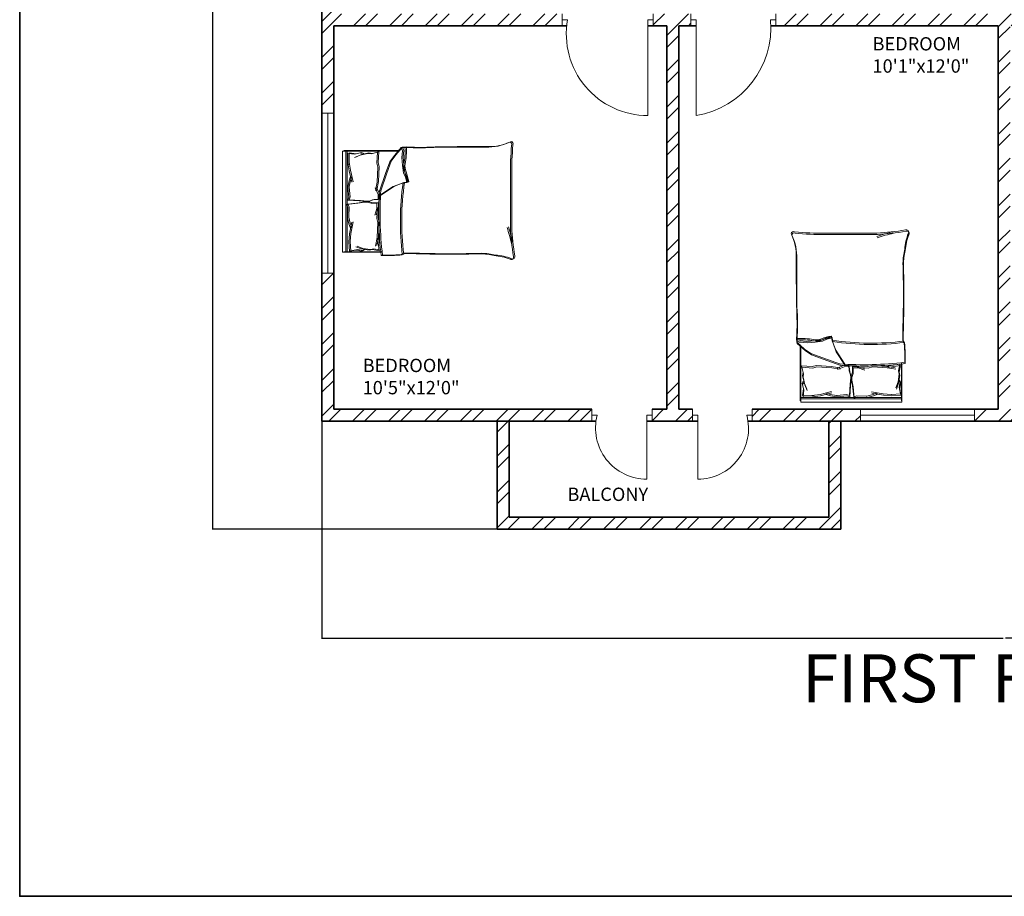
# Model space of a CAD drawing. Units: inches. Extents: x 1944 to 3454, y 1352 to 3055.
# Tile 1 of 17: x 1944 to 2314, y 1352 to 1681. Entities that reach past the tile are written whole.
import ezdxf

# ---------------------------------------------------------------- set-up
doc = ezdxf.new("R2010")
doc.units = ezdxf.units.IN
for name, color, linetype, lineweight in [('A-ANNO-DIMS', 2, 'Continuous', 18), ('A-ANNO-TITL', 7, 'Continuous', 30), ('A-ANNO-TTLB', 7, 'Continuous', 35), ('A-AREA-IDEN', 7, 'Continuous', 18), ('A-DOOR', 3, 'Continuous', 20), ('A-FURN', 8, 'Continuous', 13), ('A-GLAZ', 4, 'Continuous', 18), ('A-WALL', 7, 'Continuous', 35), ('A-WALL-PATT', 252, 'Continuous', 13)]:
    doc.layers.add(name, color=color, linetype=linetype, lineweight=lineweight)
doc.styles.get("Standard").update_dxf_attribs({"font": 'arial.ttf'})
doc.dimstyles.get("Standard").update_dxf_attribs({"dimtxt": 0.18, "dimasz": 0.18, "dimexe": 0.18, "dimexo": 0.0625, "dimgap": 0.09, "dimtad": 0, "dimtih": 1, "dimtoh": 1, "dimdec": 4, "dimzin": 0, "dimdsep": 46, "dimtxsty": 'Standard', "dimcen": 0.09, "dimadec": 0, "dimazin": 0, "dimtfac": 1, "dimtdec": 4, "dimtofl": 0, "dimtmove": 0, "dimatfit": 3, "dimfxl": 1, "dimtolj": 1, "dimtzin": 0, "dimarcsym": 0})

# ---------------------------------------------------------------- blocks, each defined once
blk = doc.blocks.new('BED-WITH-PILLOWS-01')
for p, q in [((0, 40.75), (21.15, 40.75)), ((0, 40.75), (21.15, 40.75)), ((0, 2.76), (0, 40.75)), ((0.51, 40.93), (21.66, 40.93)), ((0.51, 40.93), (21.66, 40.93)), ((1.22, 2.76), (1.22, 40.75)), ((1.22, 2.76), (1.22, 40.75)), ((1.73, 2.94), (1.73, 40.93)), ((1.73, 2.94), (1.73, 40.93)), ((22.05, 42.02), (19.47, 39.08)), ((22.05, 42.02), (19.47, 39.08)), ((22.56, 42.21), (19.98, 39.26)), ((22.56, 42.21), (19.98, 39.26)), ((23.44, 42.09), (22.05, 42.02, 3.08)), ((23.44, 42.09), (22.05, 42.02, 3.08)), ((22.55, 40.8), (22.05, 42.02)), ((22.55, 40.8), (22.05, 42.02)), ((22.3, 38.34), (22.55, 40.8)), ((22.3, 38.34), (22.55, 40.8)), ((23.95, 42.27), (22.56, 42.21, 3.08)), ((23.95, 42.27), (22.56, 42.21, 3.08)), ((23.05, 40.98), (22.56, 42.21)), ((23.05, 40.98), (22.56, 42.21)), ((22.81, 38.52), (23.05, 40.98)), ((22.81, 38.52), (23.05, 40.98)), ((2.03, 39.83), (1.96, 35.54)), ((2.03, 39.83), (1.96, 35.54)), ((2.03, 39.83), (4.58, 39.53)), ((2.03, 39.83), (4.58, 39.53)), ((2.54, 40.01), (2.46, 35.72)), ((2.54, 40.01), (2.46, 35.72)), ((2.54, 40.01), (5.09, 39.71)), ((2.54, 40.01), (5.09, 39.71)), ((6.56, 39.2), (4.43, 38.26)), ((6.56, 39.2), (4.43, 38.26)), ((4.58, 39.53), (6.63, 40.01)), ((4.58, 39.53), (6.63, 40.01)), ((7.07, 39.38), (4.94, 38.44)), ((7.07, 39.38), (4.94, 38.44)), ((5.09, 39.71), (7.14, 40.19)), ((5.09, 39.71), (7.14, 40.19)), ((9.4, 39.83), (6.56, 39.2)), ((9.4, 39.83), (6.56, 39.2)), ((6.63, 40.01), (7.46, 39.6)), ((6.63, 40.01), (7.46, 39.6)), ((9.91, 40.01), (7.07, 39.38)), ((9.91, 40.01), (7.07, 39.38)), ((7.14, 40.19), (7.97, 39.78)), ((7.14, 40.19), (7.97, 39.78)), ((10.68, 39.68), (9.4, 39.83)), ((10.68, 39.68), (9.4, 39.83)), ((11.19, 39.86), (9.91, 40.01)), ((11.19, 39.86), (9.91, 40.01)), ((13.17, 40.3), (10.68, 39.68)), ((13.17, 40.3), (10.68, 39.68)), ((13.68, 40.48), (11.19, 39.86)), ((13.68, 40.48), (11.19, 39.86)), ((12.85, 36.22), (13.17, 40.3)), ((12.85, 36.22), (13.17, 40.3)), ((13.36, 36.4), (13.68, 40.48)), ((13.36, 36.4), (13.68, 40.48)), ((19.47, 39.08), (17.75, 36.74)), ((19.47, 39.08), (17.75, 36.74)), ((19.98, 39.26), (18.26, 36.92)), ((19.98, 39.26), (18.26, 36.92)), ((22.55, 35.26), (22.3, 38.34)), ((22.55, 35.26), (22.3, 38.34)), ((23.05, 35.44), (22.81, 38.52)), ((23.05, 35.44), (22.81, 38.52)), ((1.96, 35.54), (2.02, 36.34)), ((1.96, 35.54), (2.02, 36.34)), ((2.02, 36.34), (2.44, 33.32)), ((2.02, 36.34), (2.44, 33.32)), ((2.44, 33.32), (3.51, 29.01)), ((2.44, 33.32), (3.51, 29.01)), ((2.46, 35.72), (2.53, 36.52)), ((2.46, 35.72), (2.53, 36.52)), ((2.53, 36.52), (2.95, 33.5)), ((2.53, 36.52), (2.95, 33.5)), ((2.95, 33.5), (4.02, 29.19)), ((2.95, 33.5), (4.02, 29.19)), ((13.3, 34.66), (12.85, 36.22)), ((13.3, 34.66), (12.85, 36.22)), ((12.95, 29.09), (13.3, 34.66)), ((12.95, 29.09), (13.3, 34.66)), ((13.8, 34.84), (13.36, 36.4)), ((13.8, 34.84), (13.36, 36.4)), ((13.46, 29.27), (13.8, 34.84)), ((13.46, 29.27), (13.8, 34.84)), ((17.75, 36.74), (16.15, 32.31)), ((17.75, 36.74), (16.15, 32.31)), ((18.26, 36.92), (16.66, 32.49)), ((18.26, 36.92), (16.66, 32.49)), ((22.92, 32.55), (22.55, 35.26)), ((22.92, 32.55), (22.55, 35.26)), ((23.42, 32.74), (23.05, 35.44)), ((23.42, 32.74), (23.05, 35.44)), ((2.92, 31.16), (2.45, 29.52)), ((2.92, 31.16), (2.45, 29.52)), ((2.95, 29.7), (2.52, 27.37)), ((2.95, 29.7), (2.52, 27.37)), ((3.43, 31.34), (2.95, 29.7)), ((3.43, 31.34), (2.95, 29.7)), ((16.15, 32.31), (13.82, 25.68)), ((16.15, 32.31), (13.82, 25.68)), ((16.66, 32.49), (14.33, 25.86)), ((16.66, 32.49), (14.33, 25.86)), ((23.65, 30.95), (22.92, 32.55)), ((23.65, 30.95), (22.92, 32.55)), ((24.16, 31.13), (23.42, 32.74)), ((24.16, 31.13), (23.42, 32.74)), ((24.15, 28.98), (23.65, 30.95)), ((24.15, 28.98), (23.65, 30.95)), ((24.65, 29.17), (24.16, 31.13)), ((24.65, 29.16), (24.16, 31.13)), ((62.99, 11.97), (62.99, 31.54)), ((62.99, 11.97), (62.99, 31.54)), ((63.5, 12.16), (63.5, 31.72)), ((63.5, 12.15), (63.5, 31.72)), ((2.45, 29.52), (2.02, 27.19)), ((2.45, 29.52), (2.02, 27.19)), ((2.02, 27.19), (2.03, 26.93)), ((2.02, 27.19), (2.03, 26.93)), ((2.03, 26.93), (2.37, 23.41)), ((2.03, 26.93), (2.37, 23.41)), ((2.52, 27.37), (2.54, 27.12)), ((2.52, 27.37), (2.54, 27.11)), ((2.54, 27.12), (2.88, 23.6)), ((2.54, 27.11), (2.88, 23.6)), ((13.31, 24.44), (12.28, 26.88)), ((13.31, 24.44), (12.28, 26.88)), ((12.42, 25.88), (12.95, 29.09)), ((12.42, 25.88), (12.95, 29.09)), ((13.81, 24.62), (12.79, 27.07)), ((13.81, 24.62), (12.79, 27.06)), ((12.93, 26.07), (13.46, 29.27)), ((12.93, 26.07), (13.46, 29.27)), ((13.82, 24.05), (18.98, 27.38)), ((13.82, 24.05), (18.98, 27.38)), ((14.33, 24.23), (19.49, 27.56)), ((14.33, 24.23), (19.49, 27.56)), ((18.98, 27.38), (22.55, 28.74)), ((18.98, 27.38), (22.55, 28.74)), ((19.49, 27.56), (23.05, 28.92)), ((19.49, 27.56), (23.05, 28.92)), ((22.55, 28.74), (24.15, 28.98)), ((22.55, 28.74), (24.15, 28.98)), ((23.05, 28.92), (24.65, 29.17)), ((23.05, 28.92), (24.65, 29.16)), ((2.37, 23.41), (1.98, 22.24)), ((2.37, 23.41), (1.98, 22.24)), ((1.98, 22.24), (6.25, 22.04)), ((1.98, 22.24), (6.25, 22.04)), ((2.88, 23.6), (2.49, 22.42)), ((2.88, 23.6), (2.49, 22.42)), ((2.49, 22.42), (6.76, 22.23)), ((2.49, 22.42), (6.76, 22.23)), ((6.76, 22.23), (9.31, 21.93)), ((6.76, 22.23), (9.31, 21.93)), ((9.84, 21.81), (11.3, 22.36)), ((9.84, 21.81), (11.3, 22.36)), ((10.35, 21.99), (11.81, 22.54)), ((10.35, 21.99), (11.81, 22.54)), ((11.3, 22.36), (13.43, 22.49)), ((11.3, 22.36), (13.43, 22.49)), ((11.81, 22.54), (13.94, 22.67)), ((11.81, 22.54), (13.94, 22.67)), ((13.43, 22.49), (13.31, 24.44)), ((13.43, 22.49), (13.31, 24.44)), ((13.94, 22.67), (13.81, 24.62)), ((13.94, 22.67), (13.81, 24.62)), ((1.49, 20.65), (5.74, 21.11)), ((1.49, 20.65), (5.74, 21.11)), ((1.95, 19.5), (1.49, 20.65)), ((1.95, 19.5), (1.49, 20.65)), ((1.83, 15.97), (1.95, 19.5)), ((1.83, 15.97), (1.95, 19.5)), ((1.99, 20.83), (6.25, 21.29)), ((1.99, 20.83), (6.25, 21.29)), ((2.45, 19.69), (1.99, 20.83)), ((2.45, 19.69), (1.99, 20.83)), ((2.34, 16.15), (2.45, 19.69)), ((2.34, 16.15), (2.45, 19.69)), ((5.74, 21.11), (8.27, 21.57)), ((5.74, 21.11), (8.27, 21.57)), ((6.25, 22.04), (8.81, 21.74)), ((6.25, 22.04), (8.81, 21.74)), ((6.25, 21.29), (8.78, 21.75)), ((6.25, 21.29), (8.78, 21.75)), ((8.27, 21.57), (9.3, 21.57)), ((8.27, 21.57), (9.3, 21.57)), ((8.78, 21.75), (9.81, 21.75)), ((8.78, 21.75), (9.81, 21.75)), ((8.81, 21.74), (9.84, 21.81)), ((8.81, 21.74), (9.84, 21.81)), ((9.3, 21.57), (10.8, 21.11)), ((9.3, 21.57), (10.8, 21.11)), ((9.31, 21.93), (10.35, 21.99)), ((9.31, 21.93), (10.35, 21.99)), ((9.81, 21.75), (11.3, 21.29)), ((9.81, 21.75), (11.3, 21.29)), ((10.8, 21.11), (12.93, 21.11)), ((10.8, 21.11), (12.93, 21.11)), ((11.3, 21.29), (13.44, 21.29)), ((11.3, 21.29), (13.44, 21.29)), ((12.93, 19.16), (12.06, 16.66)), ((12.93, 19.16), (12.06, 16.66)), ((13.44, 19.34), (12.57, 16.84)), ((13.44, 19.34), (12.57, 16.84)), ((12.85, 15.41), (13.17, 19.49)), ((12.85, 15.41), (13.17, 19.49)), ((12.93, 21.11), (12.93, 19.16)), ((12.93, 21.11), (12.93, 19.16)), ((13.36, 15.59), (13.68, 19.67)), ((13.36, 15.59), (13.68, 19.67)), ((13.44, 21.29), (13.44, 19.34)), ((13.44, 21.29), (13.44, 19.34)), ((1.83, 15.71), (1.83, 15.97)), ((1.83, 15.71), (1.83, 15.97)), ((2.41, 13.42), (1.83, 15.71)), ((2.41, 13.42), (1.83, 15.71)), ((2.34, 15.9), (2.34, 16.15)), ((2.34, 15.9), (2.34, 16.15)), ((2.91, 13.6), (2.34, 15.9)), ((2.91, 13.6), (2.34, 15.9)), ((13.3, 13.85), (12.85, 15.41)), ((13.3, 13.85), (12.85, 15.41)), ((13.8, 14.03), (13.36, 15.59)), ((13.8, 14.03), (13.36, 15.59)), ((2.98, 11.81), (2.41, 13.42)), ((2.98, 11.81), (2.41, 13.42)), ((2.64, 9.62), (3.44, 13.99)), ((2.64, 9.62), (3.44, 13.99)), ((3.49, 11.99), (2.91, 13.6)), ((3.49, 11.99), (2.91, 13.6)), ((3.14, 9.81), (3.95, 14.17)), ((3.14, 9.81), (3.95, 14.17)), ((12.95, 8.28), (13.3, 13.85)), ((12.95, 8.28), (13.3, 13.85)), ((13.46, 8.46), (13.8, 14.03)), ((13.46, 8.46), (13.8, 14.03)), ((2.41, 6.59), (2.64, 9.62)), ((2.41, 6.59), (2.64, 9.62)), ((2.91, 6.77), (3.14, 9.81)), ((2.91, 6.77), (3.14, 9.81)), ((12.42, 5.07), (12.95, 8.28)), ((12.42, 5.07), (12.95, 8.28)), ((12.93, 5.25), (13.46, 8.46)), ((12.93, 5.25), (13.46, 8.46)), ((12.95, 8.28), (13.21, 7.38)), ((12.95, 8.28), (13.21, 7.38)), ((13.46, 8.46), (13.72, 7.56)), ((13.46, 8.46), (13.72, 7.56)), ((13.72, 7.56), (14.29, 3.51)), ((13.72, 7.56), (14.29, 3.51)), ((2.39, 6.5), (2.41, 6.59)), ((2.39, 6.5), (2.41, 6.59)), ((2.65, 3.1), (2.39, 6.5)), ((2.65, 3.1), (2.39, 6.5)), ((2.9, 6.68), (2.91, 6.77)), ((2.9, 6.68), (2.91, 6.77)), ((3.16, 3.28), (2.9, 6.68)), ((3.16, 3.28), (2.9, 6.68)), ((3.14, 3.28), (5.67, 3.74)), ((3.14, 3.28), (5.67, 3.74)), ((7.12, 4.02), (4.93, 4.82)), ((7.12, 4.01), (4.93, 4.82)), ((7.63, 4.2), (5.44, 5)), ((7.63, 4.2), (5.44, 5)), ((5.67, 3.74), (7.74, 3.39)), ((5.67, 3.74), (7.74, 3.39)), ((9.99, 3.56), (7.12, 4.02)), ((9.99, 3.56), (7.12, 4.01)), ((10.5, 3.74), (7.63, 4.2)), ((10.5, 3.74), (7.63, 4.2)), ((7.74, 3.39), (8.55, 3.85)), ((7.74, 3.39), (8.55, 3.85)), ((11.26, 3.79), (9.99, 3.56)), ((11.26, 3.79), (9.99, 3.56)), ((11.76, 3.97), (10.5, 3.74)), ((11.76, 3.97), (10.5, 3.74)), ((13.78, 3.33), (11.26, 3.79)), ((13.78, 3.33), (11.26, 3.79)), ((14.29, 3.51), (11.76, 3.97)), ((14.29, 3.51), (11.76, 3.97)), ((13.21, 7.38), (13.78, 3.33)), ((13.21, 7.38), (13.78, 3.33)), ((14.4, 2.76), (0, 2.76)), ((14.4, 2.76), (0, 2.76)), ((14.9, 2.94), (0.51, 2.94)), ((14.9, 2.94), (0.51, 2.94)), ((2.64, 3.1), (5.16, 3.56)), ((2.64, 3.1), (5.16, 3.56)), ((5.16, 3.56), (7.23, 3.21)), ((5.16, 3.56), (7.23, 3.21)), ((7.23, 3.21), (8.04, 3.67)), ((7.23, 3.21), (8.04, 3.67))]:
    blk.add_line(p, q)
for centre, radius, start, end in [((-5.29, 40.8), 28.76, 349.8763, 2.5657), ((-5.29, 40.8), 28.76, 349.8763, 2.5657), ((28.87, 144.88), 102.94, 266.9791, 273.8365), ((28.87, 144.88), 102.94, 266.9791, 273.8365), ((-4.78, 40.98), 28.76, 349.8763, 2.5657), ((-4.78, 40.98), 28.76, 349.8763, 2.5657), ((29.37, 145.06), 102.94, 266.9791, 273.8365), ((29.37, 145.06), 102.94, 266.9791, 273.8365), ((53.91, -3583.94), 3626.16, 90.00217, 90.28689), ((53.91, -3583.94), 3626.16, 90.00217, 90.28689), ((54.42, -3583.76), 3626.16, 90.00217, 90.28689), ((54.42, -3583.76), 3626.16, 90.00217, 90.28689), ((54.58, 60.54), 18.33, 267.4714, 296.4681), ((54.58, 60.54), 18.33, 267.4714, 296.4681), ((55.09, 60.72), 18.33, 267.4714, 296.4681), ((55.09, 60.72), 18.33, 267.4714, 296.4681), ((62.69, 43.25), 0.876, 332.6588, 86.02), ((62.69, 43.25), 0.876, 332.6588, 86.02), ((168.74, 32.71), 105.75, 174.4998, 180.6351), ((168.74, 32.71), 105.75, 174.4998, 180.6351), ((63.2, 43.43), 0.876, 332.6588, 86.02), ((63.2, 43.43), 0.876, 332.6588, 86.02), ((169.24, 32.89), 105.75, 174.4998, 180.6351), ((169.24, 32.89), 105.75, 174.4998, 180.6351), ((27.87, 34.77), 4.95, 168.6608, 203.7384), ((27.87, 34.77), 4.95, 168.6608, 203.7384), ((28.38, 34.95), 4.95, 168.6608, 203.7384), ((28.38, 34.95), 4.95, 168.6608, 203.7384), ((1.18, 24.76), 23.57, 10.6617, 19.8806), ((1.18, 24.76), 23.57, 10.6617, 19.8806), ((1.69, 24.95), 23.57, 10.6617, 19.8806), ((1.69, 24.94), 23.57, 10.6617, 19.8806), ((144.71, 16.98), 131.13, 176.0865, 186.7821), ((144.71, 16.98), 131.13, 176.0865, 186.7821), ((145.22, 17.16), 131.13, 176.0865, 186.7821), ((145.22, 17.16), 131.13, 176.0865, 186.7821), ((124.25, 14.11), 102.56, 171.7845, 186.9006), ((124.25, 14.11), 102.56, 171.7845, 186.9006), ((124.76, 14.3), 102.56, 171.7845, 186.9006), ((124.76, 14.3), 102.56, 171.7845, 186.9006), ((24.2, 29.12), 0.147, 250.2464, 1.1377), ((24.2, 29.12), 0.147, 250.2464, 1.1377), ((24.7, 29.3), 0.147, 250.2464, 1.1377), ((24.7, 29.3), 0.147, 250.2464, 1.1377), ((-18.85, -13.69), 84.62, 13.3832, 17.7053), ((-18.85, -13.69), 84.62, 13.3832, 17.7053), ((-18.34, -13.51), 84.62, 13.3832, 17.7053), ((-18.34, -13.51), 84.62, 13.3832, 17.7053), ((159.64, 17.03), 96.78, 182.9958, 189.4091), ((159.64, 17.03), 96.78, 182.9958, 189.4091), ((160.15, 17.21), 96.78, 182.9958, 189.4091), ((160.15, 17.21), 96.78, 182.9958, 189.4091), ((15.97, 67.69), 66.22, 268.7218, 275.604), ((15.97, 67.69), 66.22, 268.7218, 275.604), ((16.48, 67.88), 66.22, 268.7218, 275.604), ((16.48, 67.88), 66.22, 268.7218, 275.604), ((24.78, -132.99), 135.22, 88.4762, 91.0082), ((24.78, -132.99), 135.22, 88.4762, 91.0082), ((25.29, -132.81), 135.22, 88.4762, 91.0082), ((25.29, -132.81), 135.22, 88.4762, 91.0082), ((40.23, 385.38), 383.38, 268.2277, 271.7185), ((40.23, 385.38), 383.38, 268.2277, 271.7185), ((40.74, 385.56), 383.38, 268.2277, 271.7185), ((40.74, 385.56), 383.38, 268.2277, 271.7185), ((51.28, -21.38), 23.56, 76.0648, 88.9113), ((51.28, -21.38), 23.56, 76.0648, 88.9113), ((51.79, -21.2), 23.56, 76.0648, 88.9113), ((51.79, -21.2), 23.56, 76.0648, 88.9113), ((55.86, -17.22), 18.73, 67.9751, 86.652), ((55.86, -17.22), 18.73, 67.9751, 86.652), ((56.37, -17.04), 18.73, 67.9751, 86.652), ((56.37, -17.04), 18.73, 67.9751, 86.652), ((63.37, 0.86), 0.866, 236.1736, 23.4781), ((63.37, 0.86), 0.866, 236.1736, 23.4781), ((63.87, 1.05), 0.866, 236.1736, 23.4781), ((63.87, 1.05), 0.866, 236.1736, 23.4781)]:
    blk.add_arc(centre, radius, start, end)
blk = doc.blocks.new('DOOR-SWING-36IN-07')
for p, q in [((0, 38.25), (0, 33.75)), ((34.17, 33.75), (34.17, 38.25)), ((34.17, 38.25), (34.17, 36)), ((0, 33.75), (0, 36)), ((0, 36), (2, 36)), ((34.17, 36), (32.17, 36)), ((32.17, 36), (32.17, 0))]:
    blk.add_line(p, q)
blk.add_arc((32.17, 30.64), 30.64, 169.9223, 270)
blk = doc.blocks.new('DOOR-SWING-36IN-08')
for p, q in [((0, 33.75), (0, 38.25)), ((0, 38.25), (0, 38.25)), ((0, 38.25), (0, 36)), ((31.9, 38.25), (31.9, 33.75)), ((0, 36), (2, 36)), ((2, 36), (2, 0)), ((31.9, 36), (29.9, 36)), ((31.9, 33.75), (31.9, 36))]:
    blk.add_line(p, q)
blk.add_arc((-3.46, 33.05), 33.5, 279.3869, 5.0549)
blk = doc.blocks.new('DOOR-SWING-24IN-09')
for p, q in [((0, 21.75), (0, 26.25)), ((0, 26.25), (0, 24)), ((22.65, 26.25), (22.65, 21.75)), ((0, 24), (2, 24)), ((22.65, 24), (20.65, 24)), ((20.65, 24), (20.65, 0)), ((22.65, 21.75), (22.65, 24)), ((22.65, 21.75), (22.65, 21.75))]:
    blk.add_line(p, q)
blk.add_arc((20.65, 19.25), 19.25, 165.7058, 270)
blk = doc.blocks.new('DOOR-SWING-24IN-10')
for p, q in [((0, 26.25), (0, 21.75)), ((22.35, 21.75), (22.35, 26.25)), ((22.35, 26.25), (22.35, 24)), ((0, 21.75), (0, 24)), ((0, 24), (2, 24)), ((2, 24), (2, 0)), ((22.35, 24), (20.35, 24))]:
    blk.add_line(p, q)
blk.add_arc((2, 19.01), 19.01, 270, 15.2011)
blk = doc.blocks.new('WINDOW-PLAN-60.00IN-02')
for p, q in [((2.25, 60), (0, 60)), ((0, 60), (4.5, 60)), ((2.25, 0), (2.25, 60)), ((0, 0), (4.5, 0)), ((4.5, 0), (2.25, 0))]:
    blk.add_line(p, q)
blk = doc.blocks.new('WINDOW-PLAN-42.86IN-01')
for p, q in [((0, 4.5), (0, 0)), ((42.86, 2.25), (42.86, 4.5)), ((42.86, 4.5), (42.86, 0)), ((0, 0), (0, 2.25)), ((0, 2.25), (42.86, 2.25))]:
    blk.add_line(p, q)
blk = doc.blocks.new('*D184')
at = {"layer": 'A-ANNO-DIMS', "color": 0, "lineweight": -2, "transparency": 16777216}
for p, q in [((2057.32, 1530.03), (2057.32, 1448.47)), ((2569.82, 1530.03), (2569.82, 1448.47)), ((2057.5, 1448.65), (2313.18, 1448.65)), ((2569.64, 1448.65), (2313.97, 1448.65))]:
    blk.add_line(p, q, dxfattribs=at)
at = {"layer": 'A-ANNO-DIMS', "color": 0, "transparency": 16777216}
for points in [[(2057.5, 1448.68), (2057.5, 1448.62), (2057.32, 1448.65)], [(2569.64, 1448.68), (2569.64, 1448.62), (2569.82, 1448.65)]]:
    blk.add_solid(points, dxfattribs=at)
at = {"layer": 'Defpoints', "color": 0, "transparency": 16777216}
for p in [(2057.32, 1530.1), (2569.82, 1530.1), (2569.82, 1448.65)]:
    blk.add_point(p, dxfattribs=at)
at = {"layer": 'A-ANNO-DIMS', "color": 0, "transparency": 16777216, "insert": (2313.57, 1448.65), "char_height": 0.18, "attachment_point": 5}
blk.add_mtext('\\A1;512.5', dxfattribs=at)
blk = doc.blocks.new('*D185')
at = {"layer": 'A-ANNO-DIMS', "color": 0, "lineweight": -2, "transparency": 16777216}
for p, q in [((2122.1, 2222.6), (2016.19, 2222.6)), ((2016.37, 2222.42), (2016.37, 1856.28)), ((2016.37, 1489.78), (2016.37, 1855.91)), ((2123.11, 1489.6), (2016.19, 1489.6))]:
    blk.add_line(p, q, dxfattribs=at)
at = {"layer": 'A-ANNO-DIMS', "color": 0, "transparency": 16777216}
for points in [[(2016.34, 2222.42), (2016.4, 2222.42), (2016.37, 2222.6)], [(2016.34, 1489.78), (2016.4, 1489.78), (2016.37, 1489.6)]]:
    blk.add_solid(points, dxfattribs=at)
at = {"layer": 'Defpoints', "color": 0, "transparency": 16777216}
for p in [(2016.37, 2222.6), (2122.17, 2222.6), (2123.17, 1489.6)]:
    blk.add_point(p, dxfattribs=at)
at = {"layer": 'A-ANNO-DIMS', "color": 0, "transparency": 16777216, "insert": (2016.37, 1856.1), "char_height": 0.18, "attachment_point": 5}
blk.add_mtext('\\A1;733', dxfattribs=at)

msp = doc.modelspace()

# ---------------------------------------------------------------- hatches: boundary and pattern name
at = {"layer": 'A-WALL-PATT'}
h = msp.add_hatch(dxfattribs=at)
h.set_pattern_fill('ANSI32', color=256)
h.paths.add_polyline_path([(2061.822, 2177.596), (2158.181, 2177.596), (2158.181, 2179.846), (2158.181, 2182.096), (2057.322, 2182.096), (2057.322, 2123.452), (2061.822, 2123.452)])
h.paths.add_polyline_path([(2258.993, 2179.846), (2258.993, 2182.096), (2218.838, 2182.096), (2218.838, 2177.596), (2258.993, 2177.596)])
h.paths.add_polyline_path([(2315.822, 2177.596), (2322.722, 2177.596), (2322.722, 2182.096), (2303.186, 2182.096), (2303.186, 2177.596), (2311.322, 2177.596), (2311.322, 2033.596), (2231.355, 2033.596), (2231.355, 2029.096), (2311.322, 2029.096), (2311.322, 1904.596), (2307.941, 1904.596), (2307.941, 1900.096), (2319.277, 1900.096), (2319.277, 1902.346), (2319.277, 1904.596), (2315.822, 1904.596), (2315.822, 2029.096), (2394.855, 2029.096), (2394.855, 2033.596), (2315.822, 2033.596)])
h.paths.add_polyline_path([(2407.334, 2182.096), (2366.1, 2182.096), (2366.1, 2177.596), (2407.334, 2177.596), (2407.334, 2179.846)])
h.paths.add_polyline_path([(2440.322, 2177.596), (2443.866, 2177.596), (2443.866, 2182.096), (2431.827, 2182.096), (2431.827, 2179.846), (2431.827, 2177.596), (2435.822, 2177.596), (2435.822, 2033.596), (2430.464, 2033.596), (2430.464, 2029.096), (2445.372, 2029.096), (2445.372, 2031.346), (2445.372, 2033.596), (2440.322, 2033.596)])
h.paths.add_polyline_path([(2569.822, 2182.096), (2466.481, 2182.096), (2466.481, 2177.596), (2565.322, 2177.596), (2565.322, 2123.452), (2569.822, 2123.452)])
h.paths.add_polyline_path([(2569.822, 2063.452), (2567.572, 2063.452), (2565.322, 2063.452), (2565.322, 2033.596), (2478.08, 2033.596), (2476.822, 2033.596), (2476.822, 2028.698), (2476.822, 2020.069), (2481.322, 2020.069), (2481.322, 2029.096), (2565.322, 2029.096), (2565.322, 2014.5), (2569.822, 2014.5)])
h.paths.add_polyline_path([(2569.822, 1978.5), (2565.322, 1978.5), (2565.322, 1957.096), (2481.322, 1957.096), (2481.322, 1990.369), (2476.822, 1990.369), (2476.822, 1957.096), (2476.822, 1952.596), (2476.822, 1947.471), (2481.322, 1947.471), (2481.322, 1952.596), (2565.322, 1952.596), (2565.322, 1943.2), (2569.822, 1943.2)])
h.paths.add_polyline_path([(2569.822, 1919.2), (2565.322, 1919.2), (2565.322, 1904.596), (2481.322, 1904.596), (2481.322, 1928.596), (2476.822, 1928.596), (2476.822, 1904.596), (2350.518, 1904.596), (2350.518, 1900.096), (2476.822, 1900.096), (2565.322, 1900.096), (2565.322, 1895.596), (2565.322, 1887.047), (2569.822, 1887.047)])
h.paths.add_polyline_path([(2280.492, 1904.596), (2150.322, 1904.596), (2150.322, 1926.68), (2148.072, 1926.68), (2145.822, 1926.68), (2145.822, 1904.596), (2061.822, 1904.596), (2061.822, 1914.977), (2059.572, 1914.977), (2057.322, 1914.977), (2057.322, 1887.362), (2061.822, 1887.362), (2061.822, 1900.096), (2150.322, 1900.096), (2280.492, 1900.096), (2280.492, 1902.346)])
h.paths.add_polyline_path([(2150.322, 1957.096), (2150.322, 1986.22), (2145.822, 1986.22), (2145.822, 1957.096), (2061.822, 1957.096), (2061.822, 1975.678), (2057.322, 1975.678), (2057.322, 1938.977), (2061.822, 1938.977), (2061.822, 1952.596), (2145.822, 1952.596), (2145.822, 1947.985), (2150.322, 1947.985), (2150.322, 1952.596)])
h.paths.add_polyline_path([(2061.822, 2063.452), (2057.322, 2063.452), (2057.322, 2011.678), (2061.822, 2011.678), (2061.822, 2029.096), (2145.288, 2029.096), (2145.822, 2029.096), (2145.822, 2019.118), (2150.322, 2019.118), (2150.322, 2029.096), (2150.322, 2033.596), (2147.022, 2033.596), (2061.822, 2033.596)])
h.paths.add_polyline_path([(2061.822, 1835.596), (2133.822, 1835.596), (2133.822, 1794.415), (2138.322, 1794.415), (2138.322, 1835.596), (2231.726, 1835.596), (2231.726, 1840.096), (2061.822, 1840.096), (2061.822, 1851.362), (2057.322, 1851.362), (2057.322, 1810.528), (2061.822, 1810.528)])
h.paths.add_polyline_path([(2061.822, 1774.528), (2059.572, 1774.528), (2057.322, 1774.528), (2057.322, 1723.746), (2061.822, 1723.746), (2061.822, 1735.096), (2133.822, 1735.096), (2133.822, 1731.415), (2138.322, 1731.415), (2138.322, 1759.737), (2133.822, 1759.737), (2133.822, 1739.596), (2061.822, 1739.596)])
h.paths.add_polyline_path([(2061.822, 1678.596), (2147.597, 1678.596), (2147.597, 1680.846), (2147.597, 1683.096), (2138.322, 1683.096), (2138.322, 1710.66), (2136.072, 1710.66), (2133.822, 1710.66), (2133.822, 1683.096), (2061.822, 1683.096), (2061.822, 1699.746), (2057.322, 1699.746), (2057.322, 1645.751), (2061.822, 1645.751)])
h.paths.add_polyline_path([(2061.822, 1585.751), (2057.322, 1585.751), (2057.322, 1530.096), (2158.703, 1530.096), (2158.703, 1534.596), (2061.822, 1534.596)])
h.paths.add_polyline_path([(2191.322, 1678.596), (2195.889, 1678.596), (2195.889, 1683.096), (2181.763, 1683.096), (2181.763, 1680.846), (2181.763, 1678.596), (2186.822, 1678.596), (2186.822, 1534.596), (2181.354, 1534.596), (2181.354, 1530.096), (2196.54, 1530.096), (2196.54, 1532.346), (2196.54, 1534.596), (2191.322, 1534.596)])
h.paths.add_polyline_path([(2315.822, 1678.596), (2402.014, 1678.596), (2402.014, 1683.096), (2355.822, 1683.096), (2355.822, 1835.596), (2360.838, 1835.596), (2360.838, 1840.096), (2351.322, 1840.096), (2351.322, 1683.096), (2273.322, 1683.096), (2273.322, 1840.096), (2263.134, 1840.096), (2263.134, 1837.846), (2263.134, 1835.596), (2268.822, 1835.596), (2268.822, 1683.096), (2227.793, 1683.096), (2227.793, 1678.596), (2311.322, 1678.596), (2311.322, 1534.596), (2302.384, 1534.596), (2302.384, 1530.096), (2324.521, 1530.096), (2324.521, 1532.346), (2324.521, 1534.596), (2315.822, 1534.596)])
h.paths.add_polyline_path([(2440.322, 1678.596), (2443.656, 1678.596), (2443.656, 1683.096), (2432.614, 1683.096), (2432.614, 1680.846), (2432.614, 1678.596), (2435.822, 1678.596), (2435.822, 1534.596), (2440.322, 1534.596)])
h.paths.add_polyline_path([(2409.913, 1534.596), (2369.033, 1534.596), (2369.033, 1530.096), (2409.913, 1530.096)])
h.paths.add_polyline_path([(2259.529, 1532.346), (2259.529, 1534.596), (2218.889, 1534.596), (2218.889, 1532.346), (2218.889, 1530.096), (2259.529, 1530.096)])
h.paths.add_polyline_path([(2569.822, 1584.389), (2567.572, 1584.389), (2565.322, 1584.389), (2565.322, 1534.596), (2465.892, 1534.596), (2465.892, 1530.096), (2569.822, 1530.096)])
h.paths.add_polyline_path([(2505.567, 1530.096), (2501.067, 1530.096), (2501.067, 1494.096), (2381.067, 1494.096), (2381.067, 1530.096), (2376.567, 1530.096), (2376.567, 1489.596), (2381.067, 1489.596), (2505.567, 1489.596), (2505.567, 1494.096)])
h.paths.add_polyline_path([(2127.673, 1530.096), (2123.173, 1530.096), (2123.173, 1489.596), (2127.673, 1489.596), (2252.173, 1489.596), (2252.173, 1494.096), (2252.173, 1530.096), (2247.673, 1530.096), (2247.673, 1494.096), (2127.673, 1494.096)])
h.paths.add_polyline_path([(2251.167, 2222.596), (2126.667, 2222.596), (2122.167, 2222.596), (2122.167, 2182.096), (2126.667, 2182.096), (2126.667, 2218.096), (2210.667, 2218.096), (2234.667, 2218.096), (2246.667, 2218.096), (2246.667, 2182.096), (2251.167, 2182.096), (2251.167, 2218.096)])
h.paths.add_polyline_path([(2501.916, 2222.596), (2497.416, 2222.596), (2372.916, 2222.596), (2372.916, 2218.096), (2372.916, 2182.096), (2377.416, 2182.096), (2377.416, 2218.096), (2497.416, 2218.096), (2497.416, 2182.096), (2501.916, 2182.096)])
h.paths.add_polyline_path([(2569.822, 1700.442), (2565.322, 1700.442), (2565.322, 1683.096), (2493.322, 1683.096), (2493.322, 1709.096), (2488.822, 1709.096), (2488.822, 1683.096), (2475.416, 1683.096), (2475.416, 1680.846), (2475.416, 1678.596), (2488.822, 1678.596), (2565.322, 1678.596), (2565.322, 1644.389), (2569.822, 1644.389)])
h.paths.add_polyline_path([(2569.822, 1773.506), (2565.322, 1773.506), (2565.322, 1739.596), (2493.322, 1739.596), (2493.322, 1754.002), (2488.822, 1754.002), (2488.822, 1729.846), (2491.072, 1729.846), (2493.322, 1729.846), (2493.322, 1735.096), (2565.322, 1735.096), (2565.322, 1724.442), (2569.822, 1724.442)])
h.paths.add_polyline_path([(2569.822, 1851.047), (2567.572, 1851.047), (2565.322, 1851.047), (2565.322, 1840.096), (2395.039, 1840.096), (2395.039, 1837.846), (2395.039, 1835.596), (2488.822, 1835.596), (2488.822, 1798.423), (2493.322, 1798.423), (2493.322, 1835.596), (2565.322, 1835.596), (2565.322, 1809.506), (2569.822, 1809.506)])
h.paths.add_polyline_path([(2347.275, 1955.576), (2414.024, 1955.576), (2414.024, 1974.234), (2347.275, 1974.234)], flags=9)
h.paths.add_polyline_path([(2509.756, 1990.497), (2542.915, 1990.497), (2542.915, 2009.154), (2509.756, 2009.154)], flags=9)

# ---------------------------------------------------------------- linework, layer by layer
at = {"layer": 'A-ANNO-TTLB'}
msp.add_lwpolyline([(1943.914, 3054.605), (3453.633, 3054.605), (3453.633, 1351.76), (1943.914, 1351.76)], close=True, dxfattribs=at)
at = {"layer": 'A-WALL'}
for p, q in [((2057.322, 2182.096), (2057.322, 1530.096)), ((2061.822, 1678.596), (2149.283, 1678.596)), ((2061.822, 1678.596), (2061.822, 1534.596)), ((2179.763, 1678.596), (2186.822, 1678.596)), ((2186.822, 1678.596), (2186.822, 1534.596)), ((2191.322, 1678.596), (2191.322, 1534.596)), ((2191.322, 1678.596), (2197.889, 1678.596)), ((2225.916, 1678.596), (2311.322, 1678.596)), ((2311.322, 1678.596), (2311.322, 1534.596)), ((2061.822, 1534.596), (2158.703, 1534.596)), ((2181.354, 1534.596), (2186.822, 1534.596)), ((2191.322, 1534.596), (2196.54, 1534.596)), ((2218.889, 1534.596), (2311.322, 1534.596)), ((2057.322, 1530.096), (2160.27, 1530.096)), ((2123.173, 1489.596), (2123.173, 1530.096)), ((2127.673, 1530.096), (2127.673, 1494.096)), ((2179.354, 1530.096), (2198.54, 1530.096)), ((2217.356, 1530.096), (2411.349, 1530.096)), ((2247.673, 1494.096), (2247.673, 1530.096)), ((2252.173, 1530.096), (2252.173, 1494.096)), ((2127.673, 1494.096), (2247.673, 1494.096)), ((2252.173, 1494.096), (2252.173, 1489.596)), ((2127.673, 1489.596), (2123.173, 1489.596)), ((2252.173, 1489.596), (2127.673, 1489.596))]:
    msp.add_line(p, q, dxfattribs=at)

# ---------------------------------------------------------------- block references
at = {"layer": 'A-DOOR'}
for name, p in [('DOOR-SWING-36IN-07', (2147.597, 1644.846)), ('DOOR-SWING-36IN-08', (2195.889, 1644.846)), ('DOOR-SWING-24IN-09', (2158.703, 1508.346)), ('DOOR-SWING-24IN-10', (2196.54, 1508.346))]:
    msp.add_blockref(name, p, dxfattribs=at)
at = {"layer": 'A-FURN'}
msp.add_blockref('BED-WITH-PILLOWS-01', (2065.129, 1590.799), dxfattribs=at)
at = {"layer": 'A-FURN', "rotation": 90}
msp.add_blockref('BED-WITH-PILLOWS-01', (2277.879, 1537.234), dxfattribs=at)
at = {"layer": 'A-GLAZ', "extrusion": (0, 0, -1), "zscale": -1, "rotation": 180}
msp.add_blockref('WINDOW-PLAN-60.00IN-02', (-2057.322, 1645.752), dxfattribs=at)
at = {"layer": 'A-GLAZ'}
msp.add_blockref('WINDOW-PLAN-42.86IN-01', (2259.529, 1530.096), dxfattribs=at)

# ---------------------------------------------------------------- texts
at = {"layer": 'A-ANNO-TITL', "insert": (2237.641, 1442.6), "char_height": 18, "attachment_point": 1}
msp.add_mtext_dynamic_manual_height_columns('FIRST FLOOR PLAN ', width=474.17053, gutter_width=12.5, heights=[0], dxfattribs=at)
at = {"layer": 'A-AREA-IDEN', "char_height": 5, "attachment_point": 1}
for s, width, insert in [('BEDROOM\\P10\'1"x12\'0"', 122.9432, (2264.099, 1674.29)), ('BEDROOM\\P10\'5"x12\'0"', 116.53947, (2072.682, 1553.549)), ('BALCONY', 118.50767, (2149.552, 1505.176))]:
    msp.add_mtext_dynamic_manual_height_columns(s, width=width, gutter_width=12.5, heights=[0], dxfattribs=dict(at, insert=insert))

# ---------------------------------------------------------------- dimensions: what is measured, and where the dimension line sits
at = {"layer": 'A-ANNO-DIMS'}
dim = msp.add_linear_dim(base=(2016.372, 2222.596), p1=(2123.173, 1489.596), p2=(2122.167, 2222.596), angle=90, dimstyle='Standard', override={"dimdec": 0, "dimlfac": 1, "dimrnd": 0, "dimzin": 0, "dimdsep": 46, "dimlunit": 2}, dxfattribs=at)
dim.commit()
dim.dimension.update_dxf_attribs({"geometry": '*D185', "text_midpoint": (2016.372, 1856.096)})
dim = msp.add_linear_dim(base=(2569.822, 1448.646), p1=(2057.322, 1530.096), p2=(2569.822, 1530.096), dimstyle='Standard', override={"dimdec": 1, "dimlfac": 1, "dimrnd": 0, "dimzin": 0, "dimdsep": 46, "dimlunit": 2}, dxfattribs=at)
dim.commit()
dim.dimension.update_dxf_attribs({"geometry": '*D184', "text_midpoint": (2313.572, 1448.646)})

doc.saveas('drawing.dxf')
